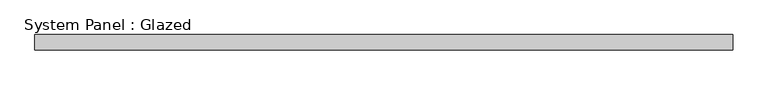
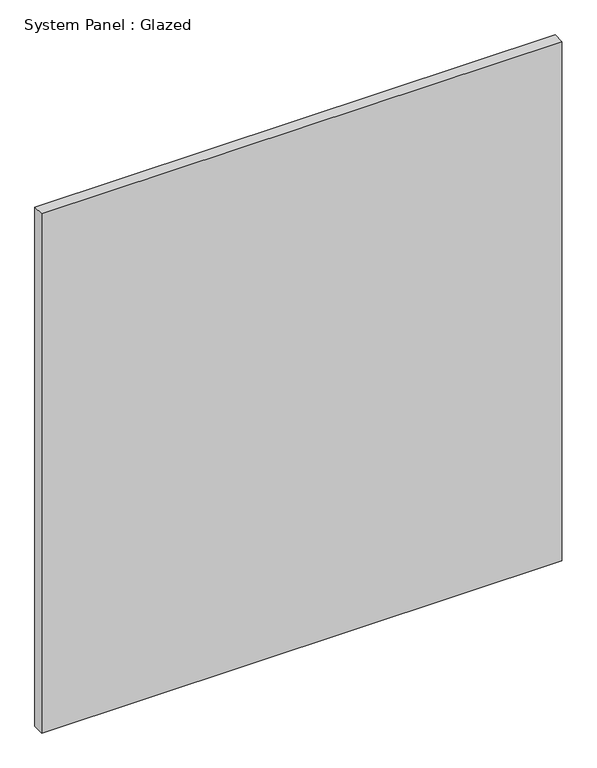
"""IFC4 building model written with IfcOpenShell, lengths in millimetres: plate geometry, System Panel : Glazed."""

from ifc_helpers import new_model, si_unit, origin, origin_with_axes, place, context, project, spatial, polyline, outline, extrude, source, transform, mapped, element, save


def system_panel_glazed_d22e8d08(model_context):
    return source(origin(), model_context, "Body", "SweptSolid", [
        extrude(outline(polyline([(572.42075, 19.05), (-572.42075, 19.05), (-572.42075, 44.45), (572.42075, 44.45), (572.42075, 19.05)])), origin_with_axes(), (0.0, 0.0, 1.0), 1208.3415),
    ])


if __name__ == "__main__":
    model = new_model("IFC4")
    model_context = context("Model", 3, world=origin())
    ifc_project = project(units=[si_unit("LENGTHUNIT", "METRE", prefix="MILLI")], contexts=[model_context])
    site = spatial("IfcSite", under=ifc_project)
    building = spatial("IfcBuilding", under=site)
    placement = place(None, origin())
    system_panel_glazed_shape = system_panel_glazed_d22e8d08(model_context)
    element("IfcPlate", 1, ObjectType="System Panel : Glazed", at=placement, inside=building, context=model_context, shape_type="MappedRepresentation", body=[
        mapped(system_panel_glazed_shape, transform((0.0, 0.0, 0.0), x_axis=(1.0, 0.0, 0.0), y_axis=(0.0, 1.0, 0.0), z_axis=(0.0, 0.0, 1.0))),
    ])
    save(model, "model.ifc")

# Revit data of these elements
# Type "System Panel : Glazed"
#   Construction Type Id = "GSP4R"
#   Analytic Construction = "1/8 in Pilkington single glazing"
#   Visual Light Transmittance = 0.9
#   Solar Heat Gain Coefficient = 0.86
#   Heat Transfer Coefficient (U) = 1.18115 BTU/(h·ft²·°F)
#   Define Thermal Properties by = 1
# Element 1 (IfcPlate, "System Panel : Glazed")
#   Materials on its faces: "Glass"
# Materials
#   "Glass": class "Glass", colour RGB 0 128 192, transparency 0.75, Description = "Soda Lime Glass", Cost = 0
